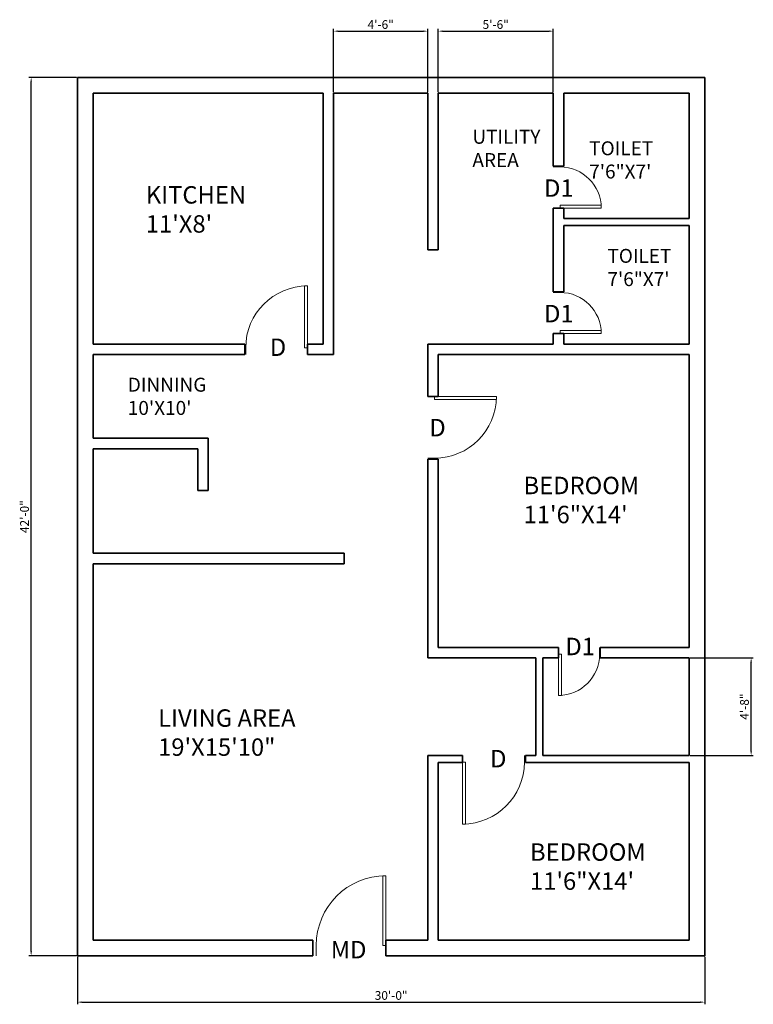
# Model space of a CAD drawing. Units: inches. Extents: x 1662 to 23131, y 1265 to 19127.
# Tile 20 of 26: x 20774 to 21195, y 18460 to 19025. Entities that reach past the tile are written whole.
import ezdxf

# ---------------------------------------------------------------- set-up
doc = ezdxf.new("R2010")
doc.units = ezdxf.units.IN
for name, color, linetype, lineweight in [('A-ANNO-DIMS', 4, 'Continuous', 18), ('A-ANNO-IDEN', 7, 'Continuous', 18), ('A-AREA-IDEN', 7, 'Continuous', 18), ('A-DOOR', 3, 'Continuous', 18), ('A-WALL', 7, 'Continuous', 35)]:
    doc.layers.add(name, color=color, linetype=linetype, lineweight=lineweight)
doc.styles.get("Standard").update_dxf_attribs({"font": 'arial.ttf'})
doc.dimstyles.new('ISO-25', dxfattribs={"dimtxt": 5, "dimasz": 2.5, "dimexe": 1.25, "dimexo": 0.625, "dimtad": 1, "dimlunit": 3, "dimtxsty": 'Standard', "dimcen": 2.5, "dimadec": 0, "dimazin": 0, "dimtfac": 1, "dimtmove": 0, "dimatfit": 3, "dimfxl": 1, "dimarcsym": 0})

# ---------------------------------------------------------------- blocks, each defined once
blk = doc.blocks.new('*U4')
for p, q in [((0, 0), (0, -100)), ((-900, 0), (-900, -100))]:
    blk.add_line(p, q)
blk.add_lwpolyline([(0, 0), (0, 900), (-43.75, 900), (-43.75, 0)], close=True)
blk.add_arc((0, 0), 900, 90, 180)
blk = doc.blocks.new('*U101')
for p, q in [((0, 0), (0, -100)), ((900, 0), (900, -100))]:
    blk.add_line(p, q)
blk.add_lwpolyline([(0, 0), (0, 900), (43.75, 900), (43.75, 0)], close=True)
blk.add_arc((0, 0), 900, 0, 90)
blk = doc.blocks.new('*U142')
for p, q in [((0, 0), (0, 100)), ((900, 0), (900, 100))]:
    blk.add_line(p, q)
blk.add_lwpolyline([(0, 0), (0, -900), (43.75, -900), (43.75, 0)], close=True)
blk.add_arc((0, 0), 900, 270, 0)
blk = doc.blocks.new('*U104')
for p, q in [((-600, 0), (-600, -100)), ((0, 0), (0, -100))]:
    blk.add_line(p, q)
blk.add_lwpolyline([(0, 0), (0, 600), (-43.75, 600), (-43.75, 0)], close=True)
blk.add_arc((0, 0), 600, 90, 180)
blk = doc.blocks.new('*U143')
for p, q in [((-600, 0), (-600, -100)), ((0, 0), (0, -100))]:
    blk.add_line(p, q)
blk.add_lwpolyline([(0, 0), (0, 600), (-43.75, 600), (-43.75, 0)], close=True)
blk.add_arc((0, 0), 600, 90, 180)
blk = doc.blocks.new('*U27')
for p, q in [((0, 0), (0, -6)), ((-40, 0), (-40, -6))]:
    blk.add_line(p, q)
blk.add_lwpolyline([(0, 0), (0, 40), (-1.75, 40), (-1.75, 0)], close=True)
blk.add_arc((0, 0), 40, 90, 180)
blk = doc.blocks.new('*D199')
at = {"layer": 'A-ANNO-DIMS', "color": 0, "lineweight": -2, "transparency": 16777216}
for p, q in [((20807.58, 18487.27), (20807.58, 18460.1)), ((21167.58, 18487.27), (21167.58, 18460.1)), ((20810.08, 18461.35), (21165.08, 18461.35))]:
    blk.add_line(p, q, dxfattribs=at)
at = {"layer": 'A-ANNO-DIMS', "color": 0, "transparency": 16777216}
for points in [[(20810.08, 18461.76), (20810.08, 18460.93), (20807.58, 18461.35)], [(21165.08, 18461.76), (21165.08, 18460.93), (21167.58, 18461.35)]]:
    blk.add_solid(points, dxfattribs=at)
at = {"layer": 'Defpoints', "color": 0, "transparency": 16777216}
for p in [(20807.58, 18487.9), (21167.58, 18487.9), (21167.58, 18461.35)]:
    blk.add_point(p, dxfattribs=at)
at = {"layer": 'A-ANNO-DIMS', "color": 0, "transparency": 16777216, "insert": (20987.58, 18464.53), "char_height": 5, "attachment_point": 5}
blk.add_mtext('30\'-0"', dxfattribs=at)
blk = doc.blocks.new('*D200')
at = {"layer": 'A-ANNO-DIMS', "color": 0, "lineweight": -2, "transparency": 16777216}
for p, q in [((20806.96, 18991.9), (20779.78, 18991.9)), ((20781.03, 18490.4), (20781.03, 18989.4)), ((20806.96, 18487.9), (20779.78, 18487.9))]:
    blk.add_line(p, q, dxfattribs=at)
at = {"layer": 'A-ANNO-DIMS', "color": 0, "transparency": 16777216}
for points in [[(20780.62, 18989.4), (20781.45, 18989.4), (20781.03, 18991.9)], [(20780.62, 18490.4), (20781.45, 18490.4), (20781.03, 18487.9)]]:
    blk.add_solid(points, dxfattribs=at)
at = {"layer": 'Defpoints', "color": 0, "transparency": 16777216}
for p in [(20781.03, 18991.9), (20807.58, 18991.9), (20807.58, 18487.9)]:
    blk.add_point(p, dxfattribs=at)
at = {"layer": 'A-ANNO-DIMS', "color": 0, "transparency": 16777216, "insert": (20777.86, 18739.9), "char_height": 5, "attachment_point": 5, "rotation": 90}
blk.add_mtext('42\'-0"', dxfattribs=at)
blk = doc.blocks.new('*D201')
at = {"layer": 'A-ANNO-DIMS', "color": 0, "lineweight": -2, "transparency": 16777216}
for p, q in [((20954.58, 18983.52), (20954.58, 19019.7)), ((20957.08, 19018.45), (21006.08, 19018.45)), ((21008.58, 18983.52), (21008.58, 19019.7))]:
    blk.add_line(p, q, dxfattribs=at)
at = {"layer": 'A-ANNO-DIMS', "color": 0, "transparency": 16777216}
for points in [[(20957.08, 19018.86), (20957.08, 19018.03), (20954.58, 19018.45)], [(21006.08, 19018.86), (21006.08, 19018.03), (21008.58, 19018.45)]]:
    blk.add_solid(points, dxfattribs=at)
at = {"layer": 'Defpoints', "color": 0, "transparency": 16777216}
for p in [(21008.58, 19018.45), (20954.58, 18982.9), (21008.58, 18982.9)]:
    blk.add_point(p, dxfattribs=at)
at = {"layer": 'A-ANNO-DIMS', "color": 0, "transparency": 16777216, "insert": (20981.58, 19021.62), "char_height": 5, "attachment_point": 5}
blk.add_mtext('4\'-6"', dxfattribs=at)
blk = doc.blocks.new('*D202')
at = {"layer": 'A-ANNO-DIMS', "color": 0, "lineweight": -2, "transparency": 16777216}
for p, q in [((21014.58, 18983.52), (21014.58, 19019.7)), ((21017.08, 19018.45), (21078.08, 19018.45)), ((21080.58, 18983.52), (21080.58, 19019.7))]:
    blk.add_line(p, q, dxfattribs=at)
at = {"layer": 'A-ANNO-DIMS', "color": 0, "transparency": 16777216}
for points in [[(21017.08, 19018.86), (21017.08, 19018.03), (21014.58, 19018.45)], [(21078.08, 19018.86), (21078.08, 19018.03), (21080.58, 19018.45)]]:
    blk.add_solid(points, dxfattribs=at)
at = {"layer": 'Defpoints', "color": 0, "transparency": 16777216}
for p in [(21080.58, 19018.45), (21014.58, 18982.9), (21080.58, 18982.9)]:
    blk.add_point(p, dxfattribs=at)
at = {"layer": 'A-ANNO-DIMS', "color": 0, "transparency": 16777216, "insert": (21047.58, 19021.62), "char_height": 5, "attachment_point": 5}
blk.add_mtext('5\'-6"', dxfattribs=at)
blk = doc.blocks.new('*D203')
at = {"layer": 'A-ANNO-DIMS', "color": 0, "lineweight": -2, "transparency": 16777216}
for p, q in [((21159.21, 18658.9), (21195.38, 18658.9)), ((21194.13, 18605.4), (21194.13, 18656.4)), ((21159.21, 18602.9), (21195.38, 18602.9))]:
    blk.add_line(p, q, dxfattribs=at)
at = {"layer": 'A-ANNO-DIMS', "color": 0, "transparency": 16777216}
for points in [[(21193.72, 18656.4), (21194.55, 18656.4), (21194.13, 18658.9)], [(21193.72, 18605.4), (21194.55, 18605.4), (21194.13, 18602.9)]]:
    blk.add_solid(points, dxfattribs=at)
at = {"layer": 'Defpoints', "color": 0, "transparency": 16777216}
for p in [(21158.58, 18658.9), (21194.13, 18658.9), (21158.58, 18602.9)]:
    blk.add_point(p, dxfattribs=at)
at = {"layer": 'A-ANNO-DIMS', "color": 0, "transparency": 16777216, "insert": (21190.96, 18630.9), "char_height": 5, "attachment_point": 5, "rotation": 90}
blk.add_mtext('4\'-8"', dxfattribs=at)

msp = doc.modelspace()

# ---------------------------------------------------------------- linework, layer by layer
at = {"layer": 'A-WALL'}
for p, q in [((20807.584, 18991.897), (21167.584, 18991.897)), ((20807.584, 18991.897), (20807.584, 18487.897)), ((21167.584, 18991.897), (21167.584, 18487.897)), ((20816.584, 18982.897), (20816.584, 18838.897)), ((20816.584, 18982.897), (20948.584, 18982.897)), ((20948.584, 18982.897), (20948.584, 18838.897)), ((20954.584, 18982.897), (20954.584, 18832.897)), ((20954.584, 18982.897), (21008.584, 18982.897)), ((21008.584, 18982.897), (21008.584, 18892.897)), ((21014.584, 18982.897), (21014.584, 18892.897)), ((21014.584, 18982.897), (21080.584, 18982.897)), ((21080.584, 18982.897), (21080.584, 18940.897)), ((21086.584, 18982.897), (21086.584, 18940.897)), ((21086.584, 18982.897), (21158.584, 18982.897)), ((21158.584, 18982.897), (21158.584, 18910.897)), ((21080.584, 18940.897), (21086.584, 18940.897)), ((21080.584, 18916.897), (21086.584, 18916.897)), ((21080.584, 18916.897), (21080.584, 18868.897)), ((21086.584, 18916.897), (21086.584, 18910.897)), ((21086.584, 18910.897), (21158.584, 18910.897)), ((21086.584, 18906.897), (21158.584, 18906.897)), ((21086.584, 18906.897), (21086.584, 18868.897)), ((21158.584, 18906.897), (21158.584, 18838.897)), ((21008.584, 18892.897), (21014.584, 18892.897)), ((21080.584, 18868.897), (21086.584, 18868.897)), ((21080.584, 18844.897), (21086.584, 18844.897)), ((21080.584, 18844.897), (21080.584, 18838.897)), ((21086.584, 18844.897), (21086.584, 18838.897)), ((20816.584, 18838.897), (20903.584, 18838.897)), ((20903.584, 18838.897), (20903.584, 18832.897)), ((20939.584, 18838.897), (20939.584, 18832.897)), ((20939.584, 18838.897), (20948.584, 18838.897)), ((21008.584, 18838.897), (21080.584, 18838.897)), ((21008.584, 18838.897), (21008.584, 18808.897)), ((21086.584, 18838.897), (21158.584, 18838.897)), ((20816.584, 18832.897), (20903.584, 18832.897)), ((20816.584, 18832.897), (20816.584, 18784.897)), ((20939.584, 18832.897), (20954.584, 18832.897)), ((21014.584, 18832.897), (21158.584, 18832.897)), ((21014.584, 18832.897), (21014.584, 18808.897)), ((21158.584, 18832.897), (21158.584, 18664.897)), ((21008.584, 18808.897), (21014.584, 18808.897)), ((20816.584, 18784.897), (20882.584, 18784.897)), ((20882.584, 18784.897), (20882.584, 18754.897)), ((20816.584, 18778.897), (20876.584, 18778.897)), ((20816.584, 18778.897), (20816.584, 18718.897)), ((20876.584, 18778.897), (20876.584, 18754.897)), ((21008.584, 18772.897), (21014.584, 18772.897)), ((21008.584, 18772.897), (21008.584, 18658.897)), ((21014.584, 18772.897), (21014.584, 18664.897)), ((20876.584, 18754.897), (20882.584, 18754.897)), ((20816.584, 18718.897), (20960.584, 18718.897)), ((20960.584, 18718.897), (20960.584, 18712.897)), ((20816.584, 18712.897), (20960.584, 18712.897)), ((20816.584, 18712.897), (20816.584, 18496.897)), ((21014.584, 18664.897), (21083.584, 18664.897)), ((21083.584, 18664.897), (21083.584, 18658.897)), ((21107.584, 18664.897), (21107.584, 18658.897)), ((21107.584, 18664.897), (21158.584, 18664.897)), ((21008.584, 18658.897), (21070.584, 18658.897)), ((21070.584, 18658.897), (21070.584, 18602.897)), ((21074.584, 18658.897), (21074.584, 18602.897)), ((21074.584, 18658.897), (21083.584, 18658.897)), ((21107.584, 18658.897), (21158.584, 18658.897)), ((21158.584, 18658.897), (21158.584, 18602.897)), ((21008.584, 18602.897), (21028.584, 18602.897)), ((21008.584, 18602.897), (21008.584, 18496.897)), ((21014.584, 18598.897), (21028.584, 18598.897)), ((21014.584, 18598.897), (21014.584, 18496.897)), ((21028.584, 18602.897), (21028.584, 18598.897)), ((21064.584, 18602.897), (21070.584, 18602.897)), ((21064.584, 18598.897), (21064.584, 18602.897)), ((21064.584, 18598.897), (21158.584, 18598.897)), ((21074.584, 18602.897), (21158.584, 18602.897)), ((21158.584, 18598.897), (21158.584, 18496.897)), ((20816.584, 18496.897), (20942.584, 18496.897)), ((20942.584, 18496.897), (20942.584, 18487.897)), ((20984.584, 18496.897), (20984.584, 18487.897)), ((20984.584, 18496.897), (21008.584, 18496.897)), ((21014.584, 18496.897), (21158.584, 18496.897)), ((20807.584, 18487.897), (20942.584, 18487.897)), ((20984.584, 18487.897), (21167.584, 18487.897))]:
    msp.add_line(p, q, dxfattribs=at)

# ---------------------------------------------------------------- block references
at = {"layer": 'A-DOOR', "xscale": 0.0393700787401575, "yscale": 0.0393700787401575, "zscale": 0.0393700787401575}
for name, p, rotation in [('*U104', (21084.521, 18916.897), 270), ('*U104', (21084.521, 18844.897), 270), ('*U101', (21012.521, 18808.897), 270), ('*U143', (21083.584, 18660.96), 180)]:
    msp.add_blockref(name, p, dxfattribs=dict(at, rotation=rotation))
for name, p in [('*U4', (20939.584, 18836.834)), ('*U142', (21028.584, 18598.96))]:
    msp.add_blockref(name, p, dxfattribs=at)
at = {"layer": 'A-DOOR'}
msp.add_blockref('*U27', (20984.584, 18493.897), dxfattribs=at)

# ---------------------------------------------------------------- texts
at = {"layer": 'A-ANNO-IDEN', "char_height": 10, "attachment_point": 1}
for s, heights, insert in [('D1', [20], (21075.323, 18933.399)), ('D1', [20], (21075.323, 18861.399)), ('D', [0], (20917.983, 18842.111)), ('D', [0], (21009.506, 18795.969)), ('D1', [20], (21087.55, 18670.397)), ('D', [0], (21044.35, 18606.027)), ('MD', [0], (20952.947, 18496.453))]:
    msp.add_mtext_dynamic_manual_height_columns(s, width=1142.59551, gutter_width=12.5, heights=heights, dxfattribs=dict(at, insert=insert))
at = {"layer": 'A-AREA-IDEN', "attachment_point": 1}
for s, insert, char_height in [('UTILITY\\PAREA', (21034.184, 18961.839), 8), ('TOILET\\P7\'6"X7\'', (21101.225, 18955.245), 8), ("KITCHEN\\P11'X8'", (20846.811, 18929.527), 10), ('TOILET\\P7\'6"X7\'', (21111.668, 18893.517), 8), ("DINNING\\P10'X10'", (20836.473, 18819.603), 8), ('BEDROOM\\P11\'6"X14\'', (21063.56, 18762.785), 10), ('LIVING AREA\\P19\'X15\'10"', (20853.875, 18629.34), 10), ('BEDROOM\\P11\'6"X14\'', (21067.257, 18552.457), 10)]:
    msp.add_mtext_dynamic_manual_height_columns(s, width=1142.59551, gutter_width=12.5, heights=[277.772], dxfattribs=dict(at, insert=insert, char_height=char_height))

# ---------------------------------------------------------------- dimensions: what is measured, and where the dimension line sits
at = {"layer": 'A-ANNO-DIMS'}
for base, p1, p2, picture, middle in [((21008.584, 19018.447), (20954.584, 18982.897), (21008.584, 18982.897), '*D201', (20981.584, 19021.625)), ((21080.584, 19018.447), (21014.584, 18982.897), (21080.584, 18982.897), '*D202', (21047.584, 19021.625)), ((21167.584, 18461.347), (20807.584, 18487.897), (21167.584, 18487.897), '*D199', (20987.584, 18464.526))]:
    dim = msp.add_linear_dim(base=base, p1=p1, p2=p2, dimstyle='ISO-25', override={"dimdec": 1, "dimlfac": 1, "dimrnd": 0, "dimzin": 1, "dimdsep": 46, "dimlunit": 4, "dimfrac": 2}, dxfattribs=at)
    dim.commit()
    dim.dimension.update_dxf_attribs({"geometry": picture, "text_midpoint": middle})
for base, p1, p2, picture, middle in [((20781.034, 18991.897), (20807.584, 18487.897), (20807.584, 18991.897), '*D200', (20777.856, 18739.897)), ((21194.134, 18658.897), (21158.584, 18602.897), (21158.584, 18658.897), '*D203', (21190.956, 18630.897))]:
    dim = msp.add_linear_dim(base=base, p1=p1, p2=p2, angle=90, dimstyle='ISO-25', override={"dimdec": 1, "dimlfac": 1, "dimrnd": 0, "dimzin": 1, "dimdsep": 46, "dimlunit": 4, "dimfrac": 2}, dxfattribs=at)
    dim.commit()
    dim.dimension.update_dxf_attribs({"geometry": picture, "text_midpoint": middle})

doc.saveas('drawing.dxf')
